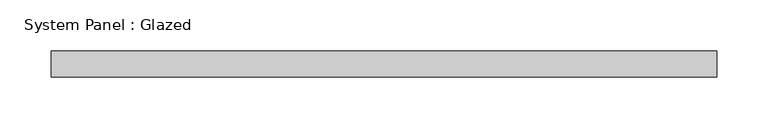
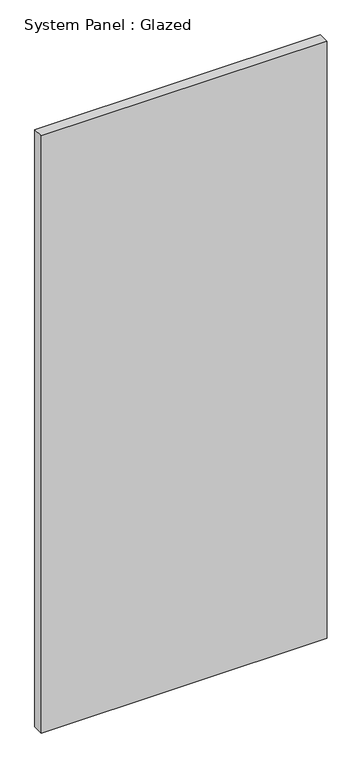
"""IFC4 building model written with IfcOpenShell, lengths in millimetres: plate geometry, System Panel : Glazed."""

from ifc_helpers import new_model, si_unit, origin, origin_with_axes, place, context, project, spatial, polyline, outline, extrude, source, transform, mapped, element, save


def system_panel_glazed_f4631ac9(model_context):
    return source(origin(), model_context, "Body", "SweptSolid", [
        extrude(outline(polyline([(323.85, 19.05), (-323.85, 19.05), (-323.85, 44.45), (323.85, 44.45), (323.85, 19.05)])), origin_with_axes(), (0.0, 0.0, 1.0), 1430.4533749),
    ])


if __name__ == "__main__":
    model = new_model("IFC4")
    model_context = context("Model", 3, world=origin())
    ifc_project = project(units=[si_unit("LENGTHUNIT", "METRE", prefix="MILLI")], contexts=[model_context])
    site = spatial("IfcSite", under=ifc_project)
    building = spatial("IfcBuilding", under=site)
    placement = place(None, origin())
    system_panel_glazed_shape = system_panel_glazed_f4631ac9(model_context)
    element("IfcPlate", 1, ObjectType="System Panel : Glazed", at=placement, inside=building, context=model_context, shape_type="MappedRepresentation", body=[
        mapped(system_panel_glazed_shape, transform((0.0, 0.0, 0.0), x_axis=(1.0, 0.0, 0.0), y_axis=(0.0, 1.0, 0.0), z_axis=(0.0, 0.0, 1.0))),
    ])
    save(model, "model.ifc")

# Revit data of these elements
# Type "System Panel : Glazed"
#   Construction Type Id = "GSP4R"
#   Analytic Construction = "1/8 in Pilkington single glazing"
#   Visual Light Transmittance = 0.9
#   Solar Heat Gain Coefficient = 0.86
#   Heat Transfer Coefficient (U) = 1.18115 BTU/(h·ft²·°F)
#   Define Thermal Properties by = 1
# Element 1 (IfcPlate, "System Panel : Glazed")
#   Materials on its faces: "Glass"
# Materials
#   "Glass": class "Glass", colour RGB 0 128 192, transparency 0.75, Description = "Soda Lime Glass", Cost = 0
